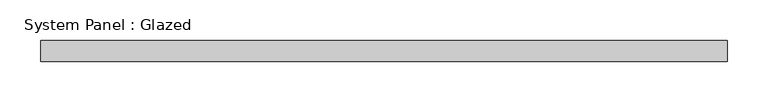
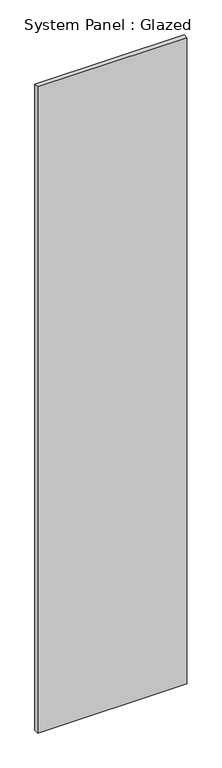
"""IFC4 building model written with IfcOpenShell, lengths in millimetres: plate geometry, System Panel : Glazed."""

from ifc_helpers import new_model, si_unit, origin, origin_with_axes, place, context, project, spatial, polyline, outline, extrude, source, transform, mapped, element, save


def system_panel_glazed_20744f22(model_context):
    return source(origin(), model_context, "Body", "SweptSolid", [
        extrude(outline(polyline([(419.1, 19.05), (-419.1, 19.05), (-419.1, 44.45), (419.1, 44.45), (419.1, 19.05)])), origin_with_axes(), (0.0, 0.0, 1.0), 3831.2450638),
    ])


if __name__ == "__main__":
    model = new_model("IFC4")
    model_context = context("Model", 3, world=origin())
    ifc_project = project(units=[si_unit("LENGTHUNIT", "METRE", prefix="MILLI")], contexts=[model_context])
    site = spatial("IfcSite", under=ifc_project)
    building = spatial("IfcBuilding", under=site)
    placement = place(None, origin())
    system_panel_glazed_shape = system_panel_glazed_20744f22(model_context)
    element("IfcPlate", 1, ObjectType="System Panel : Glazed", at=placement, inside=building, context=model_context, shape_type="MappedRepresentation", body=[
        mapped(system_panel_glazed_shape, transform((0.0, 0.0, 0.0), x_axis=(1.0, 0.0, 0.0), y_axis=(0.0, 1.0, 0.0), z_axis=(0.0, 0.0, 1.0))),
    ])
    save(model, "model.ifc")

# Revit data of these elements
# Type "System Panel : Glazed"
#   Construction Type Id = "GSP4R"
#   Analytic Construction = "1/8 in Pilkington single glazing"
#   Visual Light Transmittance = 0.9
#   Solar Heat Gain Coefficient = 0.86
#   Heat Transfer Coefficient (U) = 1.18115 BTU/(h·ft²·°F)
#   Define Thermal Properties by = 1
# Element 1 (IfcPlate, "System Panel : Glazed")
#   Materials on its faces: "Glass"
# Materials
#   "Glass": class "Glass", colour RGB 0 128 192, transparency 0.75, Description = "Soda Lime Glass", Cost = 0
